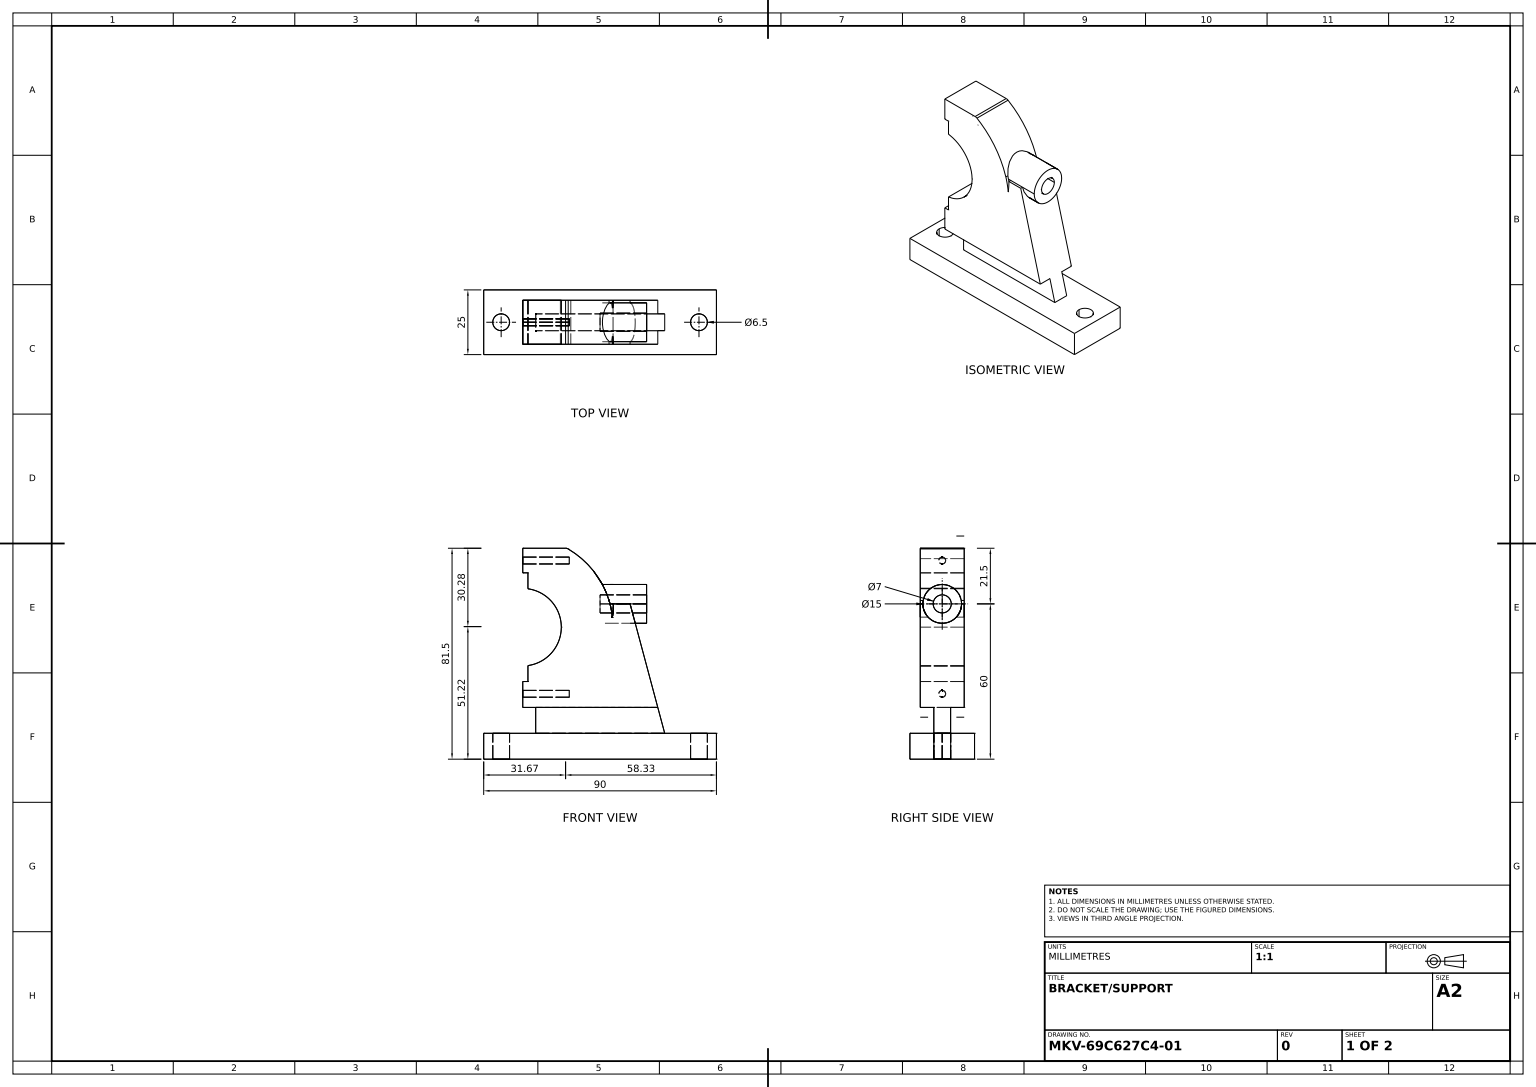
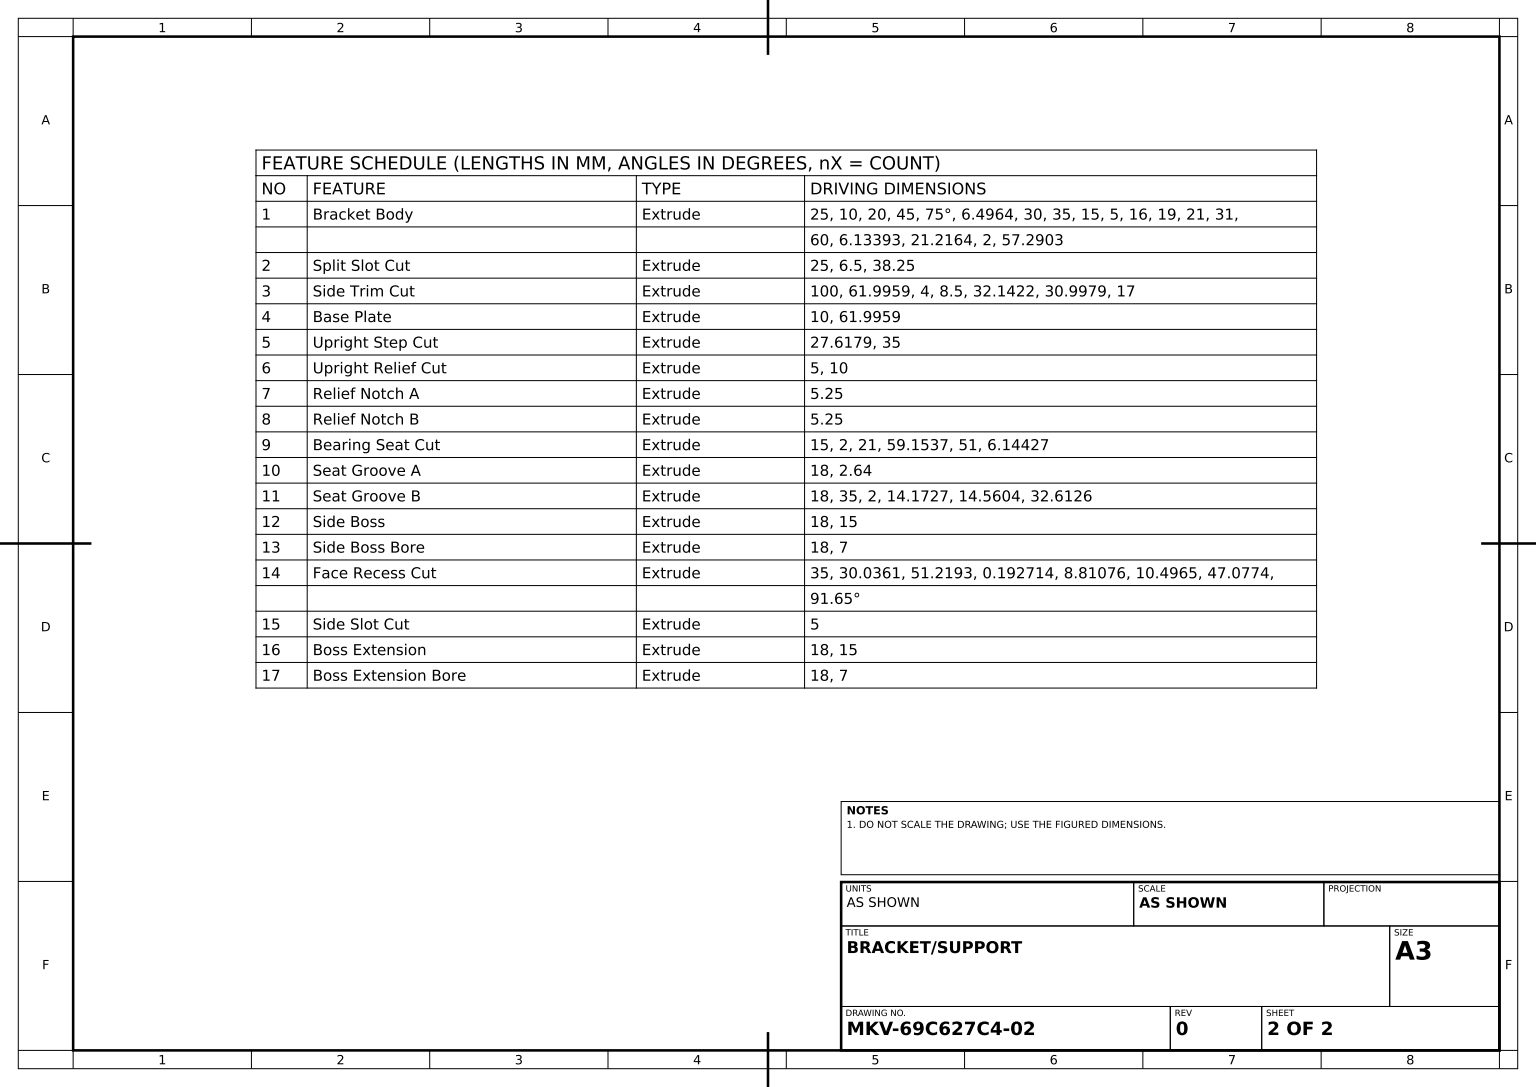
from build123d import *

# Parameters (mm, degrees)
BRACKET_PROFILE_SKETCH_W     = 5
BRACKET_PROFILE_SKETCH_H     = 10
BRACKET_BODY_DEPTH           = 12.5
SPLIT_SLOT_SKETCH_R          = 3.25
SPLIT_SLOT_CUT_DEPTH         = 25
SIDE_TRIM_SKETCH_W           = 61.995895312
SIDE_TRIM_SKETCH_H           = 4
SIDE_TRIM_CUT_DEPTH          = 100
BASE_PLATE_SKETCH_W          = 61.995895312
BASE_PLATE_SKETCH_H          = 4
BASE_PLATE_DEPTH             = 10
UPRIGHT_STEP_CUT_DEPTH       = 104.780787142
UPRIGHT_RELIEF_SKETCH_W      = 5
UPRIGHT_RELIEF_SKETCH_H      = 10
UPRIGHT_RELIEF_CUT_DEPTH     = 96.437152095
RELIEF_NOTCH_A_SKETCH_W      = 5.25
RELIEF_NOTCH_A_SKETCH_H      = 10
RELIEF_NOTCH_A_DEPTH         = 109.090938874
RELIEF_NOTCH_B_SKETCH_W      = 5.25
RELIEF_NOTCH_B_SKETCH_H      = 10
RELIEF_NOTCH_B_DEPTH         = 109.090938874
BEARING_SEAT_CUT_DEPTH       = 96.437152095
SEAT_GROOVE_A_SKETCH_R       = 1.32
SEAT_GROOVE_A_DEPTH          = 18
SEAT_GROOVE_B_DEPTH          = 18
SIDE_BOSS_SKETCH_R           = 7.5
SIDE_BOSS_DEPTH              = 18
SIDE_BOSS_BORE_SKETCH_R      = 3.5
SIDE_BOSS_BORE_DEPTH         = 18
FACE_RECESS_CUT_DEPTH        = 94.933487193
FACE_RECESS_CUT_DEPTH_BACK   = 94.933487193
SIDE_SLOT_CUT_DEPTH          = 5
BOSS_EXTENSION_SKETCH_R      = 7.5
BOSS_EXTENSION_DEPTH         = 18
BOSS_EXTENSION_BORE_SKETCH_R = 3.5
BOSS_EXTENSION_BORE_DEPTH    = 18


with BuildPart() as part:
    # Bracket Profile Sketch → Bracket Body (new, symmetric)
    with BuildSketch(Plane.XY):
        Polygon((-45, 10), (-45, 0), (0, 0), (45, 0), (45, 10), align=None)
        with BuildLine():
            Line((-13.893855715, 10), (25, 10))
            Line((25, 10), (11.602540378, 60))
            Line((11.602540378, 60), (5.106144285, 60))
            ThreePointArc((5.106144285, 60), (-0.019117223, 41.765417471), (-13.893855715, 28.871235167))
            Line((-13.893855715, 28.871235167), (-13.893855715, 10))
        make_face()
        Polygon((-24.893855715, 10), (-13.893855715, 10), (-13.893855715, 28.871235167), (-29.893855715, 29), (-29.893855715, 20), (-24.893855715, 20), align=None)
        with Locations((-27.393855715, 15)):
            Rectangle(BRACKET_PROFILE_SKETCH_W, BRACKET_PROFILE_SKETCH_H)
        with BuildLine():
            Line((-13.893855715, 41), (-13.893855715, 28.871235167))
            ThreePointArc((-13.893855715, 28.871235167), (-0.019117223, 41.765417471), (5.106144285, 60))
            ThreePointArc((5.106144285, 60), (-0.019117223, 78.234582529), (-13.893855715, 91.128764833))
            Line((-13.893855715, 91.128764833), (-13.893855715, 79))
            Line((-13.893855715, 79), (-6.677482183, 79))
            ThreePointArc((-6.677482183, 79), (0.106144285, 60), (-6.677482183, 41))
            Line((-6.677482183, 41), (-13.893855715, 41))
        make_face()
        Polygon((-29.893855715, 29), (-13.893855715, 28.871235167), (-13.893855715, 41), (-27.893855715, 41), (-27.893855715, 39), (-29.893855715, 39), align=None)
        with BuildLine():
            Line((-27.893855715, 41), (-13.893855715, 41))
            Line((-13.893855715, 41), (-13.893855715, 79))
            Line((-13.893855715, 79), (-27.893855715, 79))
            Line((-27.893855715, 79), (-27.893855715, 74.866068747))
            ThreePointArc((-27.893855715, 74.866068747), (-14.893855715, 60), (-27.893855715, 45.133931253))
            Line((-27.893855715, 45.133931253), (-27.893855715, 41))
        make_face()
        with BuildLine():
            Line((-13.893855715, 79), (-13.893855715, 41))
            Line((-13.893855715, 41), (-6.677482183, 41))
            ThreePointArc((-6.677482183, 41), (0.106144285, 60), (-6.677482183, 79))
            Line((-6.677482183, 79), (-13.893855715, 79))
        make_face()
        with BuildLine():
            Line((-29.893855715, 60), (-29.893855715, 39))
            Line((-29.893855715, 39), (-27.893855715, 39))
            Line((-27.893855715, 39), (-27.893855715, 41))
            Line((-27.893855715, 41), (-27.893855715, 45.133931253))
            ThreePointArc((-27.893855715, 45.133931253), (-14.893855715, 60), (-27.893855715, 74.866068747))
            Line((-27.893855715, 74.866068747), (-27.893855715, 79))
            Line((-27.893855715, 79), (-27.893855715, 81))
            Line((-27.893855715, 81), (-29.893855715, 81))
            Line((-29.893855715, 81), (-29.893855715, 79))
            Line((-29.893855715, 79), (-29.893855715, 60))
        make_face()
        Polygon((-13.893855715, 79), (-13.893855715, 91.128764833), (-29.893855715, 91), (-29.893855715, 81), (-27.893855715, 81), (-27.893855715, 79), align=None)
    extrude(amount=BRACKET_BODY_DEPTH, both=True)

    # Split Slot Sketch → Split Slot Cut (cut)
    with BuildSketch(Plane(origin=(0, 10, 0), x_dir=(1, 0, 0), z_dir=(0, 1, 0))):
        with Locations(Location((-38.25, 0, 0), (0, 0, 180))):
            Circle(SPLIT_SLOT_SKETCH_R)
        with Locations(Location((38.25, 0, 0), (0, 0, 270))):
            Circle(SPLIT_SLOT_SKETCH_R)
    extrude(amount=-SPLIT_SLOT_CUT_DEPTH, mode=Mode.SUBTRACT)

    # Side Trim Sketch → Side Trim Cut (cut)
    with BuildSketch(Plane(origin=(0, 0, 0), x_dir=(1, 0, 0), z_dir=(0, 1, 0))):
        with Locations((0, 10.5)):
            Rectangle(SIDE_TRIM_SKETCH_W, SIDE_TRIM_SKETCH_H)
        with Locations((0, -10.5)):
            Rectangle(SIDE_TRIM_SKETCH_W, SIDE_TRIM_SKETCH_H)
    extrude(amount=SIDE_TRIM_CUT_DEPTH, mode=Mode.SUBTRACT)

    # Base Plate Sketch → Base Plate (add)
    with BuildSketch(Plane(origin=(0, 0, 0), x_dir=(1, 0, 0), z_dir=(0, 1, 0))):
        with Locations((0, 10.5)):
            Rectangle(BASE_PLATE_SKETCH_W, BASE_PLATE_SKETCH_H)
        with Locations((0, -10.5)):
            Rectangle(BASE_PLATE_SKETCH_W, BASE_PLATE_SKETCH_H)
    extrude(amount=BASE_PLATE_DEPTH)

    # Upright Step Sketch → Upright Step Cut (cut, through all)
    with BuildSketch(Plane.XY.offset(8.5)):
        with BuildLine():
            Line((-29.893855715, 81.5), (-2.275926756, 81.5))
            ThreePointArc((-2.275926756, 81.5), (-7.559818693, 86.947927384), (-13.893855715, 91.128764833))
            Line((-13.893855715, 91.128764833), (-29.893855715, 91))
            Line((-29.893855715, 91), (-29.893855715, 81.5))
        make_face()
    extrude(amount=-UPRIGHT_STEP_CUT_DEPTH, mode=Mode.SUBTRACT)

    # Upright Relief Sketch → Upright Relief Cut (cut, through all)
    with BuildSketch(Plane.XY.offset(8.5)):
        with Locations((-27.393855715, 15)):
            Rectangle(UPRIGHT_RELIEF_SKETCH_W, UPRIGHT_RELIEF_SKETCH_H)
    extrude(amount=-UPRIGHT_RELIEF_CUT_DEPTH, mode=Mode.SUBTRACT)

    # Relief Notch A Sketch → Relief Notch A (cut, through all)
    with BuildSketch(Plane.ZY.offset(24.893855715)):
        with Locations((5.875, 15)):
            Rectangle(RELIEF_NOTCH_A_SKETCH_W, RELIEF_NOTCH_A_SKETCH_H)
    extrude(amount=-RELIEF_NOTCH_A_DEPTH, mode=Mode.SUBTRACT)

    # Relief Notch B Sketch → Relief Notch B (cut, through all)
    with BuildSketch(Plane.ZY.offset(24.893855715)):
        with Locations((-5.875, 15)):
            Rectangle(RELIEF_NOTCH_B_SKETCH_W, RELIEF_NOTCH_B_SKETCH_H)
    extrude(amount=-RELIEF_NOTCH_B_DEPTH, mode=Mode.SUBTRACT)

    # Bearing Seat Sketch → Bearing Seat Cut (cut, through all)
    with BuildSketch(Plane.XY.offset(8.5)):
        with BuildLine():
            Line((-29.969241256, 51), (-29.893855715, 30))
            Line((-29.893855715, 30), (-27.893855715, 30))
            Line((-27.893855715, 30), (-27.893855715, 36.144267946))
            ThreePointArc((-27.893855715, 36.144267946), (-14.969241256, 51), (-27.893855715, 65.855732054))
            Line((-27.893855715, 65.855732054), (-27.893855715, 72))
            Line((-27.893855715, 72), (-29.893855715, 72))
            Line((-29.893855715, 72), (-29.969241256, 51))
        make_face()
    extrude(amount=-BEARING_SEAT_CUT_DEPTH, mode=Mode.SUBTRACT)

    # Seat Groove A Sketch → Seat Groove A (cut)
    with BuildSketch(Plane.ZY.offset(29.893855715)):
        with Locations(Location((0, 76.75, 0), (0, 0, 270))):
            Circle(SEAT_GROOVE_A_SKETCH_R)
        with Locations(Location((0, 25.25, 0), (0, 0, 90))):
            Circle(SEAT_GROOVE_A_SKETCH_R)
    extrude(amount=-SEAT_GROOVE_A_DEPTH, mode=Mode.SUBTRACT)

    # Seat Groove B Sketch → Seat Groove B (cut)
    with BuildSketch(Plane.XY.offset(8.5)):
        with BuildLine():
            Line((-2.275926756, 81.5), (-13.333436496, 81.5))
            ThreePointArc((-13.333436496, 81.5), (-12.811203529, 81.430614598), (-12.325205905, 81.227272727))
            ThreePointArc((-12.325205905, 81.227272727), (-0.84803662, 70.415340341), (4.718757235, 55.662913324))
            ThreePointArc((4.718757235, 55.662913324), (3.788925867, 69.276539885), (-2.275926756, 81.5))
        make_face()
    extrude(amount=-SEAT_GROOVE_B_DEPTH, mode=Mode.SUBTRACT)

    # Side Boss Sketch → Side Boss (add)
    with BuildSketch(Plane(origin=(0, 0, 0), x_dir=(0, 0, -1), z_dir=(1, 0, 0))):
        with Locations((0, 60)):
            Circle(SIDE_BOSS_SKETCH_R)
    extrude(amount=SIDE_BOSS_DEPTH)

    # Side Boss Bore Sketch → Side Boss Bore (cut)
    with BuildSketch(Plane(origin=(18, 0, 0), x_dir=(0, 0, -1), z_dir=(1, 0, 0))):
        with Locations((0, 60)):
            Circle(SIDE_BOSS_BORE_SKETCH_R)
    extrude(amount=-SIDE_BOSS_BORE_DEPTH, mode=Mode.SUBTRACT)

    # Face Recess Sketch → Face Recess Cut (cut, two sides: drawn at the far end of the back side and taken through both)
    with BuildSketch(Plane.XY.offset(-FACE_RECESS_CUT_DEPTH_BACK)):
        with BuildLine():
            Line((-1.830885875, 81.013355064), (-12.010951395, 81.22086692))
            ThreePointArc((-12.010951395, 81.22086692), (-0.514451936, 70.02012246), (4.773427937, 54.865436626))
            ThreePointArc((4.773427937, 54.865436626), (4.090902797, 68.60104967), (-1.830885875, 81.013355064))
        make_face()
    extrude(amount=FACE_RECESS_CUT_DEPTH + FACE_RECESS_CUT_DEPTH_BACK, mode=Mode.SUBTRACT)


with BuildPart() as face_recess_cut_piece_1:
    # of the separate pieces the step leaves, piece 1, a body of its own (face_recess_cut_pieces)
    add(part.part.solids().sort_by_distance((-45, 10, -12.5))[0])

    # Boss Extension Sketch → Boss Extension (add)
    with BuildSketch(Plane(origin=(18, 0, 0), x_dir=(0, 0, -1), z_dir=(1, 0, 0))):
        with Locations((0, 60)):
            Circle(BOSS_EXTENSION_SKETCH_R)
    extrude(amount=-BOSS_EXTENSION_DEPTH)

    # Boss Extension Bore Sketch → Boss Extension Bore (cut)
    with BuildSketch(Plane(origin=(18, 0, 0), x_dir=(0, 0, -1), z_dir=(1, 0, 0))):
        with Locations((0, 60)):
            Circle(BOSS_EXTENSION_BORE_SKETCH_R)
    extrude(amount=-BOSS_EXTENSION_BORE_DEPTH, mode=Mode.SUBTRACT)


with BuildPart() as face_recess_cut_piece_2:
    # of the separate pieces the step leaves, piece 2, a body of its own (face_recess_cut_pieces)
    add(part.part.solids().sort_by_distance((-1.905011421, 81.014866049, 8.5))[0])

    # Side Slot Sketch → Side Slot Cut (cut)
    with BuildSketch(Plane(origin=(0, 0, 0), x_dir=(0, 0, -1), z_dir=(1, 0, 0))):
        Polygon((8.5, 81.5), (-8.5, 81.5), (-8.5, 81.014866049), (8.5, 81.014866049), (8.5, 81.227272727), align=None)
    extrude(amount=-SIDE_SLOT_CUT_DEPTH, mode=Mode.SUBTRACT)


solid = face_recess_cut_piece_1.part
